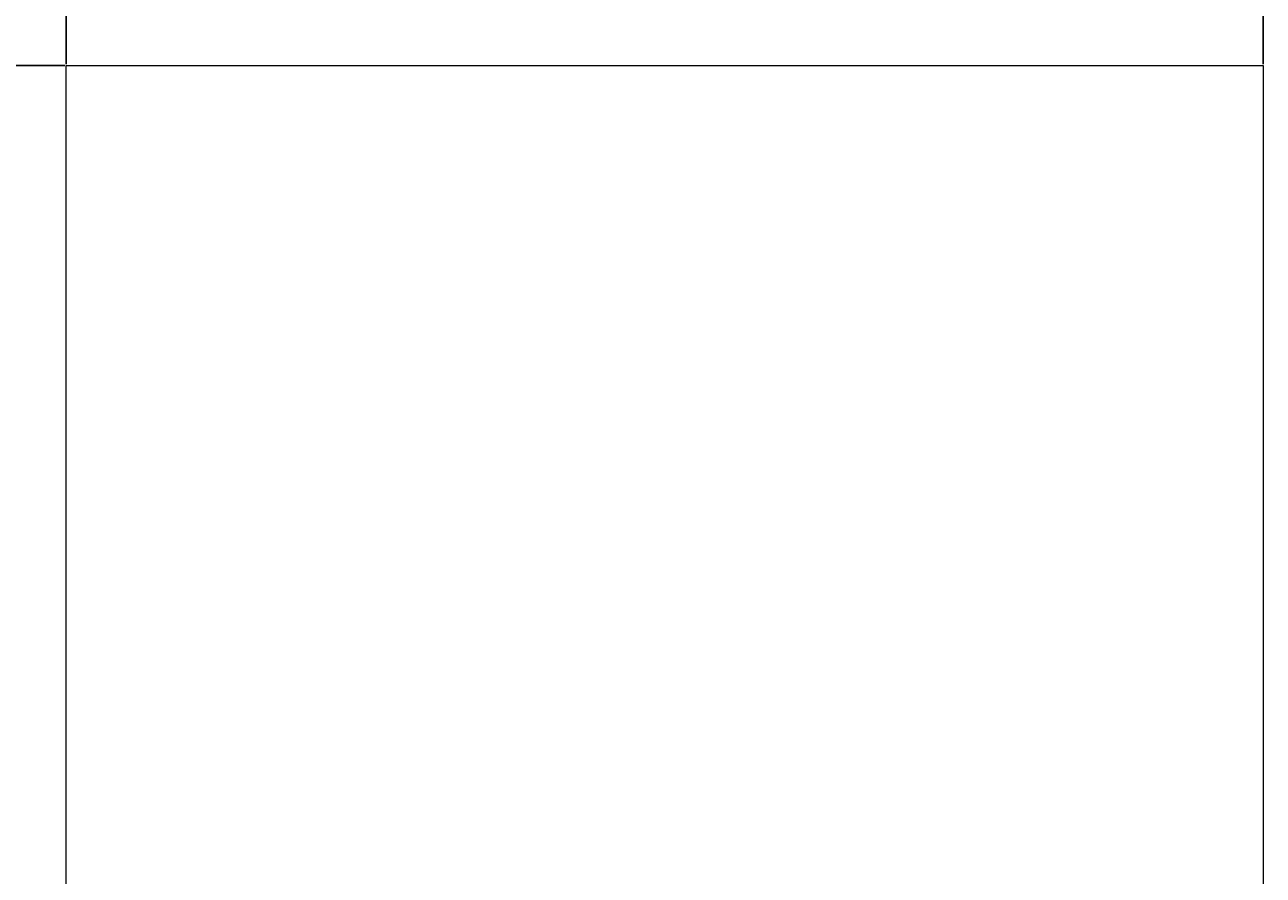
# Model space of a CAD drawing. Units: inches. Extents: x -128 to 854, y -395 to 398.
# Tile 26 of 61: x 199 to 261, y -41 to 2. Entities that reach past the tile are written whole.
import ezdxf

# ---------------------------------------------------------------- set-up
doc = ezdxf.new("R2010")
doc.units = ezdxf.units.IN
doc.header["$MEASUREMENT"] = 0
doc.layers.add('A-ANNO-DIMS', color=2, linetype='Continuous', lineweight=18)
doc.layers.add('A-FURN', color=8, linetype='Continuous', lineweight=18)
doc.styles.get("Standard").update_dxf_attribs({"font": 'arial.ttf'})
doc.dimstyles.get("Standard").update_dxf_attribs({"dimtxt": 0.18, "dimasz": 0.18, "dimexe": 0.18, "dimexo": 0.0625, "dimgap": 0.09, "dimtad": 0, "dimtih": 1, "dimtoh": 1, "dimdec": 1, "dimzin": 0, "dimdsep": 46, "dimlunit": 4, "dimtxsty": 'Standard', "dimcen": 0.09, "dimclrd": 1, "dimclre": 2, "dimclrt": 6, "dimadec": 0, "dimazin": 0, "dimtfac": 1, "dimtdec": 1, "dimtofl": 0, "dimtmove": 0, "dimatfit": 3, "dimfxl": 1, "dimtfill": 2, "dimtfillclr": 3, "dimtolj": 1, "dimtzin": 0, "dimarcsym": 0})

# ---------------------------------------------------------------- blocks, each defined once
blk = doc.blocks.new('Bed - Queen')
for p, q in [((0, -80.00003), (0, 0)), ((0, 0), (59.99999, 0)), ((59.99999, 0), (59.99999, -80.00003)), ((7.99999, -1.2), (28.79998, -1.2)), ((7.99999, -14.4), (7.99999, -1.2)), ((28.79998, -1.2), (28.79998, -14.4)), ((31.19999, -1.2), (51.99999, -1.2)), ((31.19999, -14.4), (31.19999, -1.2)), ((51.99999, -1.2), (51.99999, -16.4)), ((0, -14.4), (44.8, -14.4)), ((59.99999, -29.6), (44.8, -14.4)), ((44.8, -14.4), (44.8, -29.6)), ((51.99999, -16.4), (46.79936, -16.4)), ((44.8, -16.8), (0, -16.8)), ((44.8, -29.6), (59.99999, -29.6)), ((59.99999, -80.00003), (0, -80.00003))]:
    blk.add_line(p, q)
blk = doc.blocks.new('*D77')
at = {"layer": 'A-ANNO-DIMS', "color": 2, "lineweight": -2, "transparency": 16777216}
for p, q in [((200.764, -0.056), (188.647, -0.056)), ((200.764, -80.056), (188.647, -80.056))]:
    blk.add_line(p, q, dxfattribs=at)
at = {"layer": 'A-ANNO-DIMS', "color": 1, "lineweight": -2, "transparency": 16777216}
for p, q in [((188.827, -0.236), (188.827, -39.867)), ((188.827, -79.876), (188.827, -40.245))]:
    blk.add_line(p, q, dxfattribs=at)
at = {"layer": 'A-ANNO-DIMS', "color": 1, "transparency": 16777216}
for points in [[(188.797, -0.236), (188.857, -0.236), (188.827, -0.056)], [(188.797, -79.876), (188.857, -79.876), (188.827, -80.056)]]:
    blk.add_solid(points, dxfattribs=at)
at = {"layer": 'Defpoints', "color": 0, "transparency": 16777216}
for p in [(200.827, -0.056), (188.827, -80.056), (200.827, -80.056)]:
    blk.add_point(p, dxfattribs=at)
at = {"layer": 'A-ANNO-DIMS', "color": 6, "transparency": 16777216, "insert": (188.827, -40.056), "char_height": 0.18, "attachment_point": 5, "bg_fill": 1, "box_fill_scale": 1.25, "bg_fill_color": 3, "bg_fill_transparency": 0}
blk.add_mtext('\\A1;QUEEN BED 6\'-8" TYP.', dxfattribs=at)
blk = doc.blocks.new('*D78')
at = {"layer": 'A-ANNO-DIMS', "color": 2, "lineweight": -2, "transparency": 16777216}
for p, q in [((200.827, 0.006), (200.827, 12.124)), ((260.827, 0.006), (260.827, 12.124))]:
    blk.add_line(p, q, dxfattribs=at)
at = {"layer": 'A-ANNO-DIMS', "color": 1, "lineweight": -2, "transparency": 16777216}
for p, q in [((201.007, 11.944), (230.188, 11.944)), ((260.647, 11.944), (231.465, 11.944))]:
    blk.add_line(p, q, dxfattribs=at)
at = {"layer": 'A-ANNO-DIMS', "color": 1, "transparency": 16777216}
for points in [[(201.007, 11.974), (201.007, 11.914), (200.827, 11.944)], [(260.647, 11.974), (260.647, 11.914), (260.827, 11.944)]]:
    blk.add_solid(points, dxfattribs=at)
at = {"layer": 'Defpoints', "color": 0, "transparency": 16777216}
for p in [(200.827, 11.944), (200.827, -0.056), (260.827, -0.056)]:
    blk.add_point(p, dxfattribs=at)
at = {"layer": 'A-ANNO-DIMS', "color": 6, "transparency": 16777216, "insert": (230.827, 11.944), "char_height": 0.18, "attachment_point": 5, "bg_fill": 1, "box_fill_scale": 1.25, "bg_fill_color": 3, "bg_fill_transparency": 0}
blk.add_mtext('\\A1;5\'-0" TYP.', dxfattribs=at)

msp = doc.modelspace()

# ---------------------------------------------------------------- block references
at = {"layer": 'A-FURN', "rotation": 180}
msp.add_blockref('Bed - Queen', (260.827, -80.056), dxfattribs=at)

# ---------------------------------------------------------------- dimensions: what is measured, and where the dimension line sits
at = {"layer": 'A-ANNO-DIMS'}
for base, p1, p2, angle, text, picture, middle in [((200.827, 11.944), (260.827, -0.056), (200.827, -0.056), 180, '<> TYP.', '*D78', (230.827, 11.944)), ((188.827, -80.056), (200.827, -0.056), (200.827, -80.056), 270, 'QUEEN BED <> TYP.', '*D77', (188.827, -40.056))]:
    dim = msp.add_linear_dim(base=base, p1=p1, p2=p2, angle=angle, text=text, dimstyle='Standard', override={"dimdec": 1, "dimlfac": 1, "dimrnd": 0, "dimzin": 1, "dimdsep": 46, "dimlunit": 4, "dimfrac": 2}, dxfattribs=at)
    dim.commit()
    dim.dimension.update_dxf_attribs({"geometry": picture, "text_midpoint": middle})

doc.saveas('drawing.dxf')
